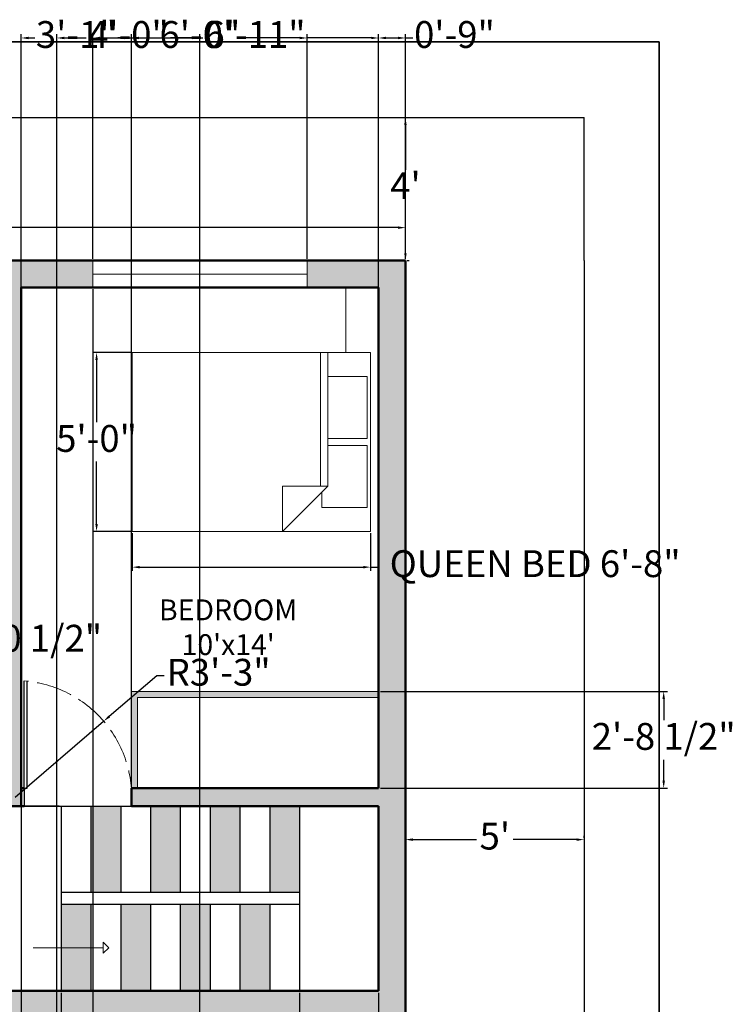
# Model space of a CAD drawing. Units: inches. Extents: x 24899 to 30135, y 37074 to 37745.
# Tile 3 of 3: x 25132 to 25371, y 37333 to 37663. Entities that reach past the tile are written whole.
import ezdxf

# ---------------------------------------------------------------- set-up
doc = ezdxf.new("R2010")
doc.units = ezdxf.units.IN
doc.linetypes.add('ACAD_ISO02W100', pattern=[15, 12, -3])
for name, color, linetype, lineweight in [('A-ANNO-DIMS', 2, 'Continuous', 18), ('A-ANNO-SYMB', 7, 'Continuous', 18), ('A-ANNO-TTLB', 7, 'Continuous', 35), ('A-AREA-IDEN', 7, 'Continuous', 25), ('A-DOOR', 4, 'Continuous', 25), ('A-DOOR-SWNG', 4, 'ACAD_ISO02W100', 13), ('A-FLOR-STRS', 7, 'Continuous', 25), ('A-FLOR-STRS-PATT', 8, 'Continuous', 13), ('A-FURN', 8, 'Continuous', 18), ('A-GLAZ', 4, 'Continuous', 18), ('A-WALL', 7, 'Continuous', 50), ('C-PROP', 3, 'Continuous', 25)]:
    doc.layers.add(name, color=color, linetype=linetype, lineweight=lineweight)
doc.layers.add('A-FURN-PATT', color=251, linetype='Continuous', lineweight=13, true_color=0x636466)
doc.layers.add('A-WALL-PATT', color=18, linetype='Continuous', lineweight=13, true_color=0x000000)
doc.styles.get("Standard").update_dxf_attribs({"font": 'arial.ttf'})
doc.dimstyles.new('ISO-25', dxfattribs={"dimtxt": 9, "dimasz": 2.5, "dimexe": 1.25, "dimexo": 0.625, "dimgap": 2, "dimtad": 0, "dimtih": 1, "dimtoh": 1, "dimdec": 1, "dimlunit": 4, "dimtxsty": 'Standard', "dimcen": 2.5, "dimadec": 0, "dimazin": 0, "dimtfac": 0.5, "dimtdec": 1, "dimtmove": 0, "dimatfit": 3, "dimfxl": 1, "dimarcsym": 0})

# ---------------------------------------------------------------- blocks, each defined once
blk = doc.blocks.new('*D1')
at = {"layer": 'A-ANNO-DIMS', "color": 0, "lineweight": -2, "transparency": 16777216}
for p, q in [((24949.48, 37583.06), (24949.48, 37594.75)), ((24951.98, 37593.5), (25095.76, 37593.5)), ((25258.98, 37593.5), (25115.19, 37593.5)), ((25261.48, 37583.06), (25261.48, 37594.75))]:
    blk.add_line(p, q, dxfattribs=at)
at = {"layer": 'A-ANNO-DIMS', "color": 0, "transparency": 16777216}
for points in [[(24951.98, 37593.92), (24951.98, 37593.09), (24949.48, 37593.5)], [(25258.98, 37593.92), (25258.98, 37593.09), (25261.48, 37593.5)]]:
    blk.add_solid(points, dxfattribs=at)
at = {"layer": 'Defpoints', "color": 0, "transparency": 16777216}
for p in [(25261.48, 37593.5), (24949.48, 37582.43), (25261.48, 37582.43)]:
    blk.add_point(p, dxfattribs=at)
at = {"layer": 'A-ANNO-DIMS', "color": 0, "transparency": 16777216, "insert": (25105.48, 37593.5), "char_height": 9, "attachment_point": 5}
blk.add_mtext("26'", dxfattribs=at)
blk = doc.blocks.new('*D7')
at = {"layer": 'A-ANNO-DIMS', "color": 0, "lineweight": -2, "transparency": 16777216}
for p, q in [((25261.48, 37388.81), (25261.48, 37389.44)), ((25263.98, 37388.19), (25285.34, 37388.19)), ((25318.98, 37388.19), (25297.62, 37388.19)), ((25321.48, 37388.81), (25321.48, 37389.44))]:
    blk.add_line(p, q, dxfattribs=at)
at = {"layer": 'A-ANNO-DIMS', "color": 0, "transparency": 16777216}
for points in [[(25263.98, 37388.6), (25263.98, 37387.77), (25261.48, 37388.19)], [(25318.98, 37388.6), (25318.98, 37387.77), (25321.48, 37388.19)]]:
    blk.add_solid(points, dxfattribs=at)
at = {"layer": 'Defpoints', "color": 0, "transparency": 16777216}
for p in [(25261.48, 37388.19), (25321.48, 37388.19), (25321.48, 37388.19)]:
    blk.add_point(p, dxfattribs=at)
at = {"layer": 'A-ANNO-DIMS', "color": 0, "transparency": 16777216, "insert": (25291.48, 37388.19), "char_height": 9, "attachment_point": 5}
blk.add_mtext("5'", dxfattribs=at)
blk = doc.blocks.new('*D8')
at = {"layer": 'A-ANNO-DIMS', "color": 0, "lineweight": -2, "transparency": 16777216}
for p, q in [((25262.1, 37630.43), (25262.73, 37630.43)), ((25261.48, 37627.93), (25261.48, 37612.93)), ((25261.48, 37584.93), (25261.48, 37599.93)), ((25262.1, 37582.43), (25262.73, 37582.43))]:
    blk.add_line(p, q, dxfattribs=at)
at = {"layer": 'A-ANNO-DIMS', "color": 0, "transparency": 16777216}
for points in [[(25261.06, 37627.93), (25261.89, 37627.93), (25261.48, 37630.43)], [(25261.06, 37584.93), (25261.89, 37584.93), (25261.48, 37582.43)]]:
    blk.add_solid(points, dxfattribs=at)
at = {"layer": 'Defpoints', "color": 0, "transparency": 16777216}
for p in [(25261.48, 37630.43), (25261.48, 37630.43), (25261.48, 37582.43)]:
    blk.add_point(p, dxfattribs=at)
at = {"layer": 'A-ANNO-DIMS', "color": 0, "transparency": 16777216, "insert": (25261.48, 37606.43), "char_height": 9, "attachment_point": 5}
blk.add_mtext("4'", dxfattribs=at)
blk = doc.blocks.new('Bed - Queen')
for p, q in [((0, -80.00003), (0, 0)), ((0, 0), (59.99999, 0)), ((59.99999, 0), (59.99999, -80.00003)), ((7.99999, -1.2), (28.79998, -1.2)), ((7.99999, -14.4), (7.99999, -1.2)), ((28.79998, -1.2), (28.79998, -14.4)), ((31.19999, -1.2), (51.99999, -1.2)), ((31.19999, -14.4), (31.19999, -1.2)), ((51.99999, -1.2), (51.99999, -16.4)), ((0, -14.4), (44.8, -14.4)), ((59.99999, -29.6), (44.8, -14.4)), ((44.8, -14.4), (44.8, -29.6)), ((51.99999, -16.4), (46.79936, -16.4)), ((44.8, -16.8), (0, -16.8)), ((44.8, -29.6), (59.99999, -29.6)), ((59.99999, -80.00003), (0, -80.00003))]:
    blk.add_line(p, q)
blk = doc.blocks.new('*D15')
at = {"layer": 'A-ANNO-DIMS', "color": 0, "lineweight": -2, "transparency": 16777216}
for p, q in [((25169.79, 37490.97), (25169.79, 37478.35)), ((25249.79, 37490.97), (25249.79, 37478.35)), ((25172.29, 37479.6), (25247.29, 37479.6)), ((25249.79, 37479.6), (25252.29, 37479.6))]:
    blk.add_line(p, q, dxfattribs=at)
at = {"layer": 'A-ANNO-DIMS', "color": 0, "transparency": 16777216}
for points in [[(25172.29, 37480.01), (25172.29, 37479.18), (25169.79, 37479.6)], [(25247.29, 37480.01), (25247.29, 37479.18), (25249.79, 37479.6)]]:
    blk.add_solid(points, dxfattribs=at)
at = {"layer": 'Defpoints', "color": 0, "transparency": 16777216}
for p in [(25169.79, 37491.6), (25249.79, 37491.6), (25249.79, 37479.6)]:
    blk.add_point(p, dxfattribs=at)
at = {"layer": 'A-ANNO-DIMS', "color": 0, "transparency": 16777216, "insert": (25305.02, 37479.6), "char_height": 9, "attachment_point": 5}
blk.add_mtext('QUEEN BED 6\'-8"', dxfattribs=at)
blk = doc.blocks.new('*D16')
at = {"layer": 'A-ANNO-DIMS', "color": 0, "lineweight": -2, "transparency": 16777216}
for p, q in [((25169.17, 37551.6), (25156.54, 37551.6)), ((25157.79, 37549.1), (25157.79, 37528.19)), ((25157.79, 37494.1), (25157.79, 37515)), ((25169.17, 37491.6), (25156.54, 37491.6))]:
    blk.add_line(p, q, dxfattribs=at)
at = {"layer": 'A-ANNO-DIMS', "color": 0, "transparency": 16777216}
for points in [[(25157.38, 37549.1), (25158.21, 37549.1), (25157.79, 37551.6)], [(25157.38, 37494.1), (25158.21, 37494.1), (25157.79, 37491.6)]]:
    blk.add_solid(points, dxfattribs=at)
at = {"layer": 'Defpoints', "color": 0, "transparency": 16777216}
for p in [(25169.79, 37551.6), (25157.79, 37491.6), (25169.79, 37491.6)]:
    blk.add_point(p, dxfattribs=at)
at = {"layer": 'A-ANNO-DIMS', "color": 0, "transparency": 16777216, "insert": (25157.79, 37521.6), "char_height": 9, "attachment_point": 5}
blk.add_mtext('5\'-0"', dxfattribs=at)
blk = doc.blocks.new('*D22')
at = {"layer": 'A-ANNO-DIMS', "color": 0, "lineweight": -2, "transparency": 16777216}
for p, q in [((25087.48, 37572.81), (25087.48, 37086.48)), ((25111.48, 37572.81), (25111.48, 37086.48)), ((25089.98, 37087.73), (25108.98, 37087.73)), ((25111.48, 37087.73), (25113.98, 37087.73))]:
    blk.add_line(p, q, dxfattribs=at)
at = {"layer": 'A-ANNO-DIMS', "color": 0, "transparency": 16777216}
for points in [[(25089.98, 37088.15), (25089.98, 37087.32), (25087.48, 37087.73)], [(25108.98, 37088.15), (25108.98, 37087.32), (25111.48, 37087.73)]]:
    blk.add_solid(points, dxfattribs=at)
at = {"layer": 'Defpoints', "color": 0, "transparency": 16777216}
for p in [(25087.48, 37573.43), (25111.48, 37573.43), (25111.48, 37087.73)]:
    blk.add_point(p, dxfattribs=at)
at = {"layer": 'A-ANNO-DIMS', "color": 0, "transparency": 16777216, "insert": (25128.02, 37087.73), "char_height": 9, "attachment_point": 5}
blk.add_mtext('2\'-0"', dxfattribs=at)
blk = doc.blocks.new('*D23')
at = {"layer": 'A-ANNO-DIMS', "color": 0, "lineweight": -2, "transparency": 16777216}
for p, q in [((25132.48, 37572.81), (25132.48, 37086.48)), ((25156.48, 37572.81), (25156.48, 37086.48)), ((25134.98, 37087.73), (25153.98, 37087.73)), ((25156.48, 37087.73), (25158.98, 37087.73))]:
    blk.add_line(p, q, dxfattribs=at)
at = {"layer": 'A-ANNO-DIMS', "color": 0, "transparency": 16777216}
for points in [[(25134.98, 37088.15), (25134.98, 37087.32), (25132.48, 37087.73)], [(25153.98, 37088.15), (25153.98, 37087.32), (25156.48, 37087.73)]]:
    blk.add_solid(points, dxfattribs=at)
at = {"layer": 'Defpoints', "color": 0, "transparency": 16777216}
for p in [(25132.48, 37573.43), (25156.48, 37573.43), (25156.48, 37087.73)]:
    blk.add_point(p, dxfattribs=at)
at = {"layer": 'A-ANNO-DIMS', "color": 0, "transparency": 16777216, "insert": (25173.02, 37087.73), "char_height": 9, "attachment_point": 5}
blk.add_mtext('2\'-0"', dxfattribs=at)
blk = doc.blocks.new('*D24')
at = {"layer": 'A-ANNO-DIMS', "color": 0, "lineweight": -2, "transparency": 16777216}
for p, q in [((25156.48, 37583.06), (25156.48, 37658.38)), ((25228.48, 37583.06), (25228.48, 37658.38)), ((25158.98, 37657.13), (25178.49, 37657.13)), ((25225.98, 37657.13), (25206.46, 37657.13))]:
    blk.add_line(p, q, dxfattribs=at)
at = {"layer": 'A-ANNO-DIMS', "color": 0, "transparency": 16777216}
for points in [[(25158.98, 37657.55), (25158.98, 37656.72), (25156.48, 37657.13)], [(25225.98, 37657.55), (25225.98, 37656.72), (25228.48, 37657.13)]]:
    blk.add_solid(points, dxfattribs=at)
at = {"layer": 'Defpoints', "color": 0, "transparency": 16777216}
for p in [(25228.48, 37657.13), (25156.48, 37582.43), (25228.48, 37582.43)]:
    blk.add_point(p, dxfattribs=at)
at = {"layer": 'A-ANNO-DIMS', "color": 0, "transparency": 16777216, "insert": (25192.48, 37657.13), "char_height": 9, "attachment_point": 5}
blk.add_mtext('6\'-0"', dxfattribs=at)
blk = doc.blocks.new('*D29')
at = {"layer": 'A-ANNO-DIMS', "color": 0, "lineweight": -2, "transparency": 16777216}
for p, q in [((25132.48, 37406.06), (25132.48, 37658.38)), ((25169.48, 37406.06), (25169.48, 37658.38)), ((25134.98, 37657.13), (25137.02, 37657.13)), ((25166.98, 37657.13), (25164.94, 37657.13))]:
    blk.add_line(p, q, dxfattribs=at)
at = {"layer": 'A-ANNO-DIMS', "color": 0, "transparency": 16777216}
for points in [[(25134.98, 37657.55), (25134.98, 37656.72), (25132.48, 37657.13)], [(25166.98, 37657.55), (25166.98, 37656.72), (25169.48, 37657.13)]]:
    blk.add_solid(points, dxfattribs=at)
at = {"layer": 'Defpoints', "color": 0, "transparency": 16777216}
for p in [(25169.48, 37657.13), (25132.48, 37405.43), (25169.48, 37405.43)]:
    blk.add_point(p, dxfattribs=at)
at = {"layer": 'A-ANNO-DIMS', "color": 0, "transparency": 16777216, "insert": (25150.98, 37657.13), "char_height": 9, "attachment_point": 5}
blk.add_mtext('3\'-1"', dxfattribs=at)
blk = doc.blocks.new('*D30')
at = {"layer": 'A-ANNO-DIMS', "color": 0, "lineweight": -2, "transparency": 16777216}
for p, q in [((25145.9, 37336.81), (25145.9, 37086.48)), ((25225.9, 37336.81), (25225.9, 37086.48)), ((25148.4, 37087.73), (25171.91, 37087.73)), ((25223.4, 37087.73), (25199.89, 37087.73))]:
    blk.add_line(p, q, dxfattribs=at)
at = {"layer": 'A-ANNO-DIMS', "color": 0, "transparency": 16777216}
for points in [[(25148.4, 37088.15), (25148.4, 37087.32), (25145.9, 37087.73)], [(25223.4, 37088.15), (25223.4, 37087.32), (25225.9, 37087.73)]]:
    blk.add_solid(points, dxfattribs=at)
at = {"layer": 'Defpoints', "color": 0, "transparency": 16777216}
for p in [(25145.9, 37337.43), (25225.9, 37337.43), (25225.9, 37087.73)]:
    blk.add_point(p, dxfattribs=at)
at = {"layer": 'A-ANNO-DIMS', "color": 0, "transparency": 16777216, "insert": (25185.9, 37087.73), "char_height": 9, "attachment_point": 5}
blk.add_mtext('6\'-8"', dxfattribs=at)
blk = doc.blocks.new('*D31')
at = {"layer": 'A-ANNO-DIMS', "color": 0, "lineweight": -2, "transparency": 16777216}
for p, q in [((25225.9, 37336.81), (25225.9, 37086.48)), ((25252.48, 37336.81), (25252.48, 37086.48)), ((25228.4, 37087.73), (25249.98, 37087.73)), ((25252.48, 37087.73), (25254.98, 37087.73))]:
    blk.add_line(p, q, dxfattribs=at)
at = {"layer": 'A-ANNO-DIMS', "color": 0, "transparency": 16777216}
for points in [[(25228.4, 37088.15), (25228.4, 37087.32), (25225.9, 37087.73)], [(25249.98, 37088.15), (25249.98, 37087.32), (25252.48, 37087.73)]]:
    blk.add_solid(points, dxfattribs=at)
at = {"layer": 'Defpoints', "color": 0, "transparency": 16777216}
for p in [(25225.9, 37337.43), (25252.48, 37337.43), (25252.48, 37087.73)]:
    blk.add_point(p, dxfattribs=at)
at = {"layer": 'A-ANNO-DIMS', "color": 0, "transparency": 16777216, "insert": (25279.5, 37087.73), "char_height": 9, "attachment_point": 5}
blk.add_mtext('2\'-2 1/2"', dxfattribs=at)
blk = doc.blocks.new('*D32')
at = {"layer": 'A-ANNO-DIMS', "color": 0, "lineweight": -2, "transparency": 16777216}
for p, q in [((25145.27, 37399.43), (24921.53, 37399.43)), ((24922.78, 37396.93), (24922.78, 37375.03)), ((24922.78, 37339.93), (24922.78, 37361.84)), ((25145.27, 37337.43), (24921.53, 37337.43))]:
    blk.add_line(p, q, dxfattribs=at)
at = {"layer": 'A-ANNO-DIMS', "color": 0, "transparency": 16777216}
for points in [[(24922.36, 37396.93), (24923.19, 37396.93), (24922.78, 37399.43)], [(24922.36, 37339.93), (24923.19, 37339.93), (24922.78, 37337.43)]]:
    blk.add_solid(points, dxfattribs=at)
at = {"layer": 'Defpoints', "color": 0, "transparency": 16777216}
for p in [(24922.78, 37399.43), (25145.9, 37399.43), (25145.9, 37337.43)]:
    blk.add_point(p, dxfattribs=at)
at = {"layer": 'A-ANNO-DIMS', "color": 0, "transparency": 16777216, "insert": (24922.78, 37368.43), "char_height": 9, "attachment_point": 5}
blk.add_mtext('5\'-2"', dxfattribs=at)
blk = doc.blocks.new('*D33')
at = {"layer": 'A-ANNO-DIMS', "color": 0, "lineweight": -2, "transparency": 16777216}
for p, q in [((25144.48, 37184.06), (25144.48, 37658.38)), ((25192.48, 37184.06), (25192.48, 37658.38)), ((25146.98, 37657.13), (25154.33, 37657.13)), ((25189.98, 37657.13), (25182.62, 37657.13))]:
    blk.add_line(p, q, dxfattribs=at)
at = {"layer": 'A-ANNO-DIMS', "color": 0, "transparency": 16777216}
for points in [[(25146.98, 37657.55), (25146.98, 37656.72), (25144.48, 37657.13)], [(25189.98, 37657.55), (25189.98, 37656.72), (25192.48, 37657.13)]]:
    blk.add_solid(points, dxfattribs=at)
at = {"layer": 'Defpoints', "color": 0, "transparency": 16777216}
for p in [(25192.48, 37657.13), (25144.48, 37183.43), (25192.48, 37183.43)]:
    blk.add_point(p, dxfattribs=at)
at = {"layer": 'A-ANNO-DIMS', "color": 0, "transparency": 16777216, "insert": (25168.48, 37657.13), "char_height": 9, "attachment_point": 5}
blk.add_mtext('4\'-0"', dxfattribs=at)
blk = doc.blocks.new('*D42')
at = {"layer": 'A-ANNO-DIMS', "color": 0, "lineweight": -2, "transparency": 16777216}
for p, q in [((25169.48, 37406.06), (25169.48, 37658.38)), ((25252.48, 37406.06), (25252.48, 37658.38)), ((25171.98, 37657.13), (25193.49, 37657.13)), ((25249.98, 37657.13), (25228.46, 37657.13))]:
    blk.add_line(p, q, dxfattribs=at)
at = {"layer": 'A-ANNO-DIMS', "color": 0, "transparency": 16777216}
for points in [[(25171.98, 37657.55), (25171.98, 37656.72), (25169.48, 37657.13)], [(25249.98, 37657.55), (25249.98, 37656.72), (25252.48, 37657.13)]]:
    blk.add_solid(points, dxfattribs=at)
at = {"layer": 'Defpoints', "color": 0, "transparency": 16777216}
for p in [(25252.48, 37657.13), (25169.48, 37405.43), (25252.48, 37405.43)]:
    blk.add_point(p, dxfattribs=at)
at = {"layer": 'A-ANNO-DIMS', "color": 0, "transparency": 16777216, "insert": (25210.98, 37657.13), "char_height": 9, "attachment_point": 5}
blk.add_mtext('6\'-11"', dxfattribs=at)
blk = doc.blocks.new('*D43')
at = {"layer": 'A-ANNO-DIMS', "color": 0, "lineweight": -2, "transparency": 16777216}
for p, q in [((25253.1, 37437.87), (25349.43, 37437.87)), ((25348.18, 37435.37), (25348.18, 37428.3)), ((25348.18, 37407.93), (25348.18, 37415)), ((25253.1, 37405.43), (25349.43, 37405.43))]:
    blk.add_line(p, q, dxfattribs=at)
at = {"layer": 'A-ANNO-DIMS', "color": 0, "transparency": 16777216}
for points in [[(25347.76, 37435.37), (25348.59, 37435.37), (25348.18, 37437.87)], [(25347.76, 37407.93), (25348.59, 37407.93), (25348.18, 37405.43)]]:
    blk.add_solid(points, dxfattribs=at)
at = {"layer": 'Defpoints', "color": 0, "transparency": 16777216}
for p in [(25252.48, 37437.87), (25348.18, 37437.87), (25252.48, 37405.43)]:
    blk.add_point(p, dxfattribs=at)
at = {"layer": 'A-ANNO-DIMS', "color": 0, "transparency": 16777216, "insert": (25348.18, 37421.65), "char_height": 9, "attachment_point": 5}
blk.add_mtext('2\'-8 1/2"', dxfattribs=at)
blk = doc.blocks.new('*D44')
at = {"layer": 'A-ANNO-DIMS', "color": 0, "lineweight": -2, "transparency": 16777216}
for p, q in [((25252.48, 37574.06), (25252.48, 37658.38)), ((25261.48, 37583.06), (25261.48, 37658.38)), ((25254.98, 37657.13), (25258.98, 37657.13)), ((25261.48, 37657.13), (25263.98, 37657.13))]:
    blk.add_line(p, q, dxfattribs=at)
at = {"layer": 'A-ANNO-DIMS', "color": 0, "transparency": 16777216}
for points in [[(25254.98, 37657.55), (25254.98, 37656.72), (25252.48, 37657.13)], [(25258.98, 37657.55), (25258.98, 37656.72), (25261.48, 37657.13)]]:
    blk.add_solid(points, dxfattribs=at)
at = {"layer": 'Defpoints', "color": 0, "transparency": 16777216}
for p in [(25261.48, 37657.13), (25261.48, 37582.43), (25252.48, 37573.43)]:
    blk.add_point(p, dxfattribs=at)
at = {"layer": 'A-ANNO-DIMS', "color": 0, "transparency": 16777216, "insert": (25277.94, 37657.13), "char_height": 9, "attachment_point": 5}
blk.add_mtext('0\'-9"', dxfattribs=at)
blk = doc.blocks.new('*D47')
at = {"layer": 'A-ANNO-DIMS', "color": 0, "lineweight": -2, "transparency": 16777216}
for p, q in [((25177.99, 37443.16), (25162.07, 37429.52)), ((25180.49, 37443.16), (25177.99, 37443.16)), ((25130.48, 37402.43), (25160.17, 37427.89))]:
    blk.add_line(p, q, dxfattribs=at)
at = {"layer": 'A-ANNO-DIMS', "color": 0, "transparency": 16777216}
blk.add_solid([(25161.8, 37429.83), (25162.34, 37429.2), (25160.17, 37427.89)], dxfattribs=at)
at = {"layer": 'Defpoints', "color": 0, "transparency": 16777216}
for p in [(25160.17, 37427.89), (25130.48, 37402.43)]:
    blk.add_point(p, dxfattribs=at)
at = {"layer": 'A-ANNO-DIMS', "color": 0, "transparency": 16777216, "insert": (25198.76, 37443.16), "char_height": 9, "attachment_point": 5}
blk.add_mtext('R3\'-3"', dxfattribs=at)
blk = doc.blocks.new('*D50')
at = {"layer": 'A-ANNO-DIMS', "color": 0, "lineweight": -2, "transparency": 16777216}
for p, q in [((25075.33, 37454.58), (25072.83, 37454.58)), ((25077.83, 37454.58), (25088.11, 37454.58)), ((25093.11, 37454.58), (25090.61, 37454.58))]:
    blk.add_line(p, q, dxfattribs=at)
at = {"layer": 'A-ANNO-DIMS', "color": 0, "transparency": 16777216}
for points in [[(25075.33, 37454.99), (25075.33, 37454.16), (25077.83, 37454.58)], [(25090.61, 37455), (25090.61, 37454.16), (25088.11, 37454.58)]]:
    blk.add_solid(points, dxfattribs=at)
at = {"layer": 'Defpoints', "color": 0, "transparency": 16777216}
for p in [(25077.83, 37454.58), (25088.11, 37454.58)]:
    blk.add_point(p, dxfattribs=at)
at = {"layer": 'A-ANNO-DIMS', "color": 0, "transparency": 16777216, "insert": (25125.95, 37454.58), "char_height": 9, "attachment_point": 5}
blk.add_mtext('∅0\'-10 1/2"', dxfattribs=at)

msp = doc.modelspace()

# ---------------------------------------------------------------- hatches: boundary and pattern name
at = {"layer": 'A-FLOR-STRS-PATT'}
h = msp.add_hatch(color=256, dxfattribs=at)
h.dxf.hatch_style = 1
h.paths.add_polyline_path([(25155.9, 37366.43), (25145.9, 37366.43), (25145.9, 37351.93), (25155.9, 37351.93)])
h.paths.add_polyline_path([(25155.9, 37351.93), (25145.9, 37351.93), (25145.9, 37337.43), (25155.9, 37337.43)])
h.paths.add_polyline_path([(25175.9, 37366.43), (25165.9, 37366.43), (25165.9, 37337.43), (25175.9, 37337.43)])
h.paths.add_polyline_path([(25195.9, 37366.43), (25185.9, 37366.43), (25185.9, 37337.43), (25195.9, 37337.43)])
h.paths.add_polyline_path([(25215.9, 37366.43), (25205.9, 37366.43), (25205.9, 37337.43), (25215.9, 37337.43)])
h.paths.add_polyline_path([(25225.9, 37399.43), (25215.9, 37399.43), (25215.9, 37370.43), (25225.9, 37370.43)])
h.paths.add_polyline_path([(25205.9, 37399.43), (25195.9, 37399.43), (25195.9, 37370.43), (25205.9, 37370.43)])
h.paths.add_polyline_path([(25185.9, 37399.43), (25175.9, 37399.43), (25175.9, 37370.43), (25185.9, 37370.43)])
h.paths.add_polyline_path([(25165.9, 37399.43), (25155.9, 37399.43), (25155.9, 37370.43), (25165.9, 37370.43)])
at = {"layer": 'A-FURN-PATT'}
h = msp.add_hatch(color=256, dxfattribs=at)
h.dxf.hatch_style = 1
h.paths.add_polyline_path([(25171.48, 37435.87), (25252.48, 37435.87), (25252.48, 37437.87), (25169.48, 37437.87), (25169.48, 37405.43), (25171.48, 37405.43)])
at = {"layer": 'A-WALL-PATT'}
h = msp.add_hatch(color=256, dxfattribs=at)
h.dxf.hatch_style = 1
h.paths.add_polyline_path([(25261.48, 37582.43), (25228.48, 37582.43), (25228.48, 37573.43), (25252.48, 37573.43), (25252.48, 37405.43), (25169.48, 37405.43, -0.038405), (25169.48, 37399.43), (25252.48, 37399.43), (25252.48, 37337.43), (25201.48, 37337.43), (24958.48, 37337.43), (24958.48, 37465.43), (24988.48, 37465.43), (24988.48, 37471.43), (24958.48, 37471.43), (24958.48, 37573.43), (24994.48, 37573.43), (24994.48, 37582.43), (24949.48, 37582.43), (24949.48, 37174.43), (25144.48, 37174.43, -0.042779), (25144.48, 37183.43), (24958.48, 37183.43), (24958.48, 37328.43), (25192.48, 37328.43), (25192.48, 37183.43), (25192.48, 37174.43), (25201.48, 37174.43), (25201.48, 37183.43), (25201.48, 37328.43), (25261.48, 37328.43)])
h.paths.add_polyline_path([(25087.48, 37582.43), (25030.48, 37582.43, -0.077125), (25030.48, 37573.43), (25066.48, 37573.43), (25066.48, 37471.43), (25036.48, 37471.43), (25036.48, 37465.43), (25066.48, 37465.43), (25066.48, 37430.04), (25095.6, 37430.04), (25095.6, 37435.01), (25072.48, 37435.01), (25072.48, 37465.43), (25072.48, 37471.43), (25095.48, 37471.43, -0.045361), (25095.48, 37477.43), (25072.48, 37477.43), (25072.48, 37573.43), (25087.48, 37573.43)], flags=0)
h.paths.add_polyline_path([(25156.48, 37582.43), (25111.48, 37582.43), (25111.48, 37573.43), (25126.48, 37573.43), (25126.48, 37477.43), (25126.48, 37471.43), (25126.48, 37399.43), (25132.48, 37399.43), (25132.48, 37405.43), (25132.48, 37471.43), (25132.48, 37573.43), (25156.48, 37573.43)], flags=17)

# ---------------------------------------------------------------- linework, layer by layer
at = {"layer": 'A-ANNO-SYMB'}
for p, q in [((25155.9, 37351.93), (25136.45, 37351.93)), ((25155.9, 37351.93), (25160.05, 37351.93)), ((25160.05, 37351.93), (25160.02, 37353.77)), ((25160.02, 37353.77), (25161.89, 37351.9)), ((25160.04, 37350.05), (25160.05, 37351.93)), ((25161.89, 37351.9), (25160.04, 37350.05))]:
    msp.add_line(p, q, dxfattribs=at)
at = {"layer": 'A-ANNO-TTLB'}
msp.add_lwpolyline([(24909.5, 37655.83), (25346.61, 37655.83), (25346.61, 37086.99), (24909.5, 37086.99)], close=True, dxfattribs=at)
at = {"layer": 'A-DOOR'}
for p, q in [((25133.48, 37405.43), (25133.48, 37441.43)), ((25134.48, 37405.43), (25134.48, 37441.43)), ((25133.48, 37405.43), (25133.48, 37399.43)), ((25133.48, 37405.43), (25134.48, 37405.43)), ((25133.48, 37399.43), (25169.48, 37399.43))]:
    msp.add_line(p, q, dxfattribs=at)
at = {"layer": 'A-DOOR-SWNG'}
msp.add_arc((25130.48, 37402.43), 39.12, 355.6013, 85.6013, dxfattribs=at)
at = {"layer": 'A-FLOR-STRS'}
for p, q in [((25145.9, 37399.43), (25145.9, 37337.43)), ((25155.9, 37399.43), (25155.9, 37370.43)), ((25165.9, 37399.43), (25165.9, 37370.43)), ((25175.9, 37399.43), (25175.9, 37370.43)), ((25185.9, 37399.43), (25185.9, 37370.43)), ((25195.9, 37399.43), (25195.9, 37370.43)), ((25205.9, 37399.43), (25205.9, 37370.43)), ((25215.9, 37399.43), (25215.9, 37370.43)), ((25225.9, 37399.43), (25225.9, 37337.43)), ((25225.9, 37370.43), (25145.9, 37370.43)), ((25225.9, 37366.43), (25145.9, 37366.43)), ((25155.9, 37366.43), (25155.9, 37337.43)), ((25165.9, 37366.43), (25165.9, 37337.43)), ((25175.9, 37366.43), (25175.9, 37337.43)), ((25185.9, 37366.43), (25185.9, 37337.43)), ((25195.9, 37366.43), (25195.9, 37337.43)), ((25205.9, 37366.43), (25205.9, 37337.43)), ((25215.9, 37366.43), (25215.9, 37337.43))]:
    msp.add_line(p, q, dxfattribs=at)
at = {"layer": 'A-FURN'}
for p, q in [((25241.52, 37573.43), (25241.52, 37551.6)), ((25252.48, 37437.87), (25169.48, 37437.87)), ((25169.48, 37405.43), (25169.48, 37437.87)), ((25252.48, 37435.87), (25171.48, 37435.87)), ((25171.48, 37405.43), (25171.48, 37435.87))]:
    msp.add_line(p, q, dxfattribs=at)
at = {"layer": 'A-GLAZ'}
for p, q in [((25156.48, 37573.43), (25156.48, 37582.43)), ((25228.48, 37573.43), (25228.48, 37582.43)), ((25156.48, 37577.93), (25228.48, 37577.93))]:
    msp.add_line(p, q, dxfattribs=at)
at = {"layer": 'A-WALL'}
for p, q in [((25030.48, 37582.43), (25261.48, 37582.43)), ((25261.48, 37328.43), (25261.48, 37582.43)), ((25132.48, 37573.43), (25132.48, 37471.43)), ((25132.48, 37573.43), (25252.48, 37573.43)), ((25252.48, 37405.43), (25252.48, 37573.43)), ((25132.48, 37471.43), (25132.48, 37405.43)), ((25132.48, 37405.43), (25133.48, 37405.43)), ((25132.48, 37405.43), (25132.48, 37399.43)), ((25169.48, 37405.43), (25169.48, 37399.43)), ((25169.48, 37405.43), (25252.48, 37405.43)), ((25132.48, 37399.43), (25126.48, 37399.43)), ((25132.48, 37399.43), (25133.48, 37399.43)), ((25169.48, 37399.43), (25252.48, 37399.43)), ((25252.48, 37337.43), (25252.48, 37399.43)), ((24958.48, 37337.43), (25201.48, 37337.43)), ((25201.48, 37337.43), (25252.48, 37337.43))]:
    msp.add_line(p, q, dxfattribs=at)
at = {"layer": 'C-PROP'}
for p, q in [((24949.48, 37630.43), (25321.48, 37630.43)), ((25321.48, 37582.43), (25321.48, 37630.43)), ((25321.48, 37582.43), (25321.48, 37114.43))]:
    msp.add_line(p, q, dxfattribs=at)

# ---------------------------------------------------------------- block references
at = {"layer": 'A-FURN', "rotation": 270}
msp.add_blockref('Bed - Queen', (25249.79, 37551.6), dxfattribs=at)

# ---------------------------------------------------------------- texts
at = {"layer": 'A-AREA-IDEN', "insert": (25167.93, 37468.77), "char_height": 7, "attachment_point": 1}
msp.add_mtext_dynamic_manual_height_columns("\\pxqc;{\\fArial|b1|i0|c0|p34;BEDROOM\\P10'x14'}", width=68.0767, gutter_width=12.5, heights=[0], dxfattribs=at)

# ---------------------------------------------------------------- dimensions: what is measured, and where the dimension line sits
at = {"layer": 'A-ANNO-DIMS'}
for base, p1, p2, override, picture, middle in [((25169.48, 37657.13), (25132.48, 37405.43), (25169.48, 37405.43), {"dimdec": 1, "dimlfac": 1, "dimrnd": 0, "dimzin": 1, "dimdsep": 46, "dimlunit": 4, "dimfrac": 2}, '*D29', (25150.98, 37657.13)), ((25192.48, 37657.13), (25144.48, 37183.43), (25192.48, 37183.43), {"dimdec": 1, "dimlfac": 1, "dimrnd": 0, "dimzin": 1, "dimdsep": 46, "dimlunit": 4, "dimfrac": 2}, '*D33', (25168.48, 37657.13)), ((25228.48, 37657.13), (25156.48, 37582.43), (25228.48, 37582.43), {"dimdec": 1, "dimlfac": 1, "dimrnd": 0, "dimzin": 1, "dimdsep": 46, "dimlunit": 4, "dimfrac": 2}, '*D24', (25192.48, 37657.13)), ((25252.48, 37657.13), (25169.48, 37405.43), (25252.48, 37405.43), {"dimdec": 1, "dimlfac": 1, "dimrnd": 0, "dimzin": 1, "dimdsep": 46, "dimlunit": 4, "dimfrac": 2}, '*D42', (25210.98, 37657.13)), ((25261.48, 37657.13), (25252.48, 37573.43), (25261.48, 37582.43), {"dimdec": 1, "dimlfac": 1, "dimrnd": 0, "dimzin": 1, "dimdsep": 46, "dimlunit": 4, "dimfrac": 2}, '*D44', (25277.94, 37657.13)), ((25261.48, 37593.5), (24949.48, 37582.43), (25261.48, 37582.43), {"dimclrd": 0, "dimclre": 0, "dimclrt": 0}, '*D1', (25105.48, 37593.5)), ((25111.48, 37087.73), (25087.48, 37573.43), (25111.48, 37573.43), {"dimdec": 1, "dimlfac": 1, "dimrnd": 0, "dimzin": 1, "dimdsep": 46, "dimlunit": 4, "dimfrac": 2}, '*D22', (25128.02, 37087.73)), ((25156.48, 37087.73), (25132.48, 37573.43), (25156.48, 37573.43), {"dimdec": 1, "dimlfac": 1, "dimrnd": 0, "dimzin": 1, "dimdsep": 46, "dimlunit": 4, "dimfrac": 2}, '*D23', (25173.02, 37087.73)), ((25225.9, 37087.73), (25145.9, 37337.43), (25225.9, 37337.43), {"dimdec": 1, "dimlfac": 1, "dimrnd": 0, "dimzin": 1, "dimdsep": 46, "dimlunit": 4, "dimfrac": 2}, '*D30', (25185.9, 37087.73)), ((25252.48, 37087.73), (25225.9, 37337.43), (25252.48, 37337.43), {"dimdec": 1, "dimlfac": 1, "dimrnd": 0, "dimzin": 1, "dimdsep": 46, "dimlunit": 4, "dimfrac": 2}, '*D31', (25279.5, 37087.73))]:
    dim = msp.add_linear_dim(base=base, p1=p1, p2=p2, dimstyle='ISO-25', override=override, dxfattribs=at)
    dim.commit()
    dim.dimension.update_dxf_attribs({"geometry": picture, "text_midpoint": middle})
for base, p1, p2, angle, override, picture, middle in [((25261.48, 37630.43), (25261.48, 37582.43), (25261.48, 37630.43), 90, {"dimclrd": 0, "dimclre": 0, "dimclrt": 0}, '*D8', (25261.48, 37606.43)), ((25157.79, 37491.6), (25169.79, 37551.6), (25169.79, 37491.6), 270, {"dimdec": 1, "dimlfac": 1, "dimrnd": 0, "dimzin": 1, "dimdsep": 46, "dimlunit": 4, "dimfrac": 2}, '*D16', (25157.79, 37521.6)), ((25348.18, 37437.87), (25252.48, 37405.43), (25252.48, 37437.87), 90, {"dimdec": 1, "dimlfac": 1, "dimrnd": 0, "dimzin": 1, "dimdsep": 46, "dimlunit": 4, "dimfrac": 2}, '*D43', (25348.18, 37421.65)), ((24922.78, 37399.43), (25145.9, 37337.43), (25145.9, 37399.43), 90, {"dimdec": 1, "dimlfac": 1, "dimrnd": 0, "dimzin": 1, "dimdsep": 46, "dimlunit": 4, "dimfrac": 2}, '*D32', (24922.78, 37368.43)), ((25321.48, 37388.19), (25261.48, 37388.19), (25321.48, 37388.19), 180, {"dimclrd": 0, "dimclre": 0, "dimclrt": 0}, '*D7', (25291.48, 37388.19))]:
    dim = msp.add_linear_dim(base=base, p1=p1, p2=p2, angle=angle, dimstyle='ISO-25', override=override, dxfattribs=at)
    dim.commit()
    dim.dimension.update_dxf_attribs({"geometry": picture, "text_midpoint": middle})
dim = msp.add_linear_dim(base=(25249.79, 37479.6), p1=(25169.79, 37491.6), p2=(25249.79, 37491.6), text='QUEEN BED <>', dimstyle='ISO-25', override={"dimdec": 1, "dimlfac": 1, "dimrnd": 0, "dimzin": 1, "dimdsep": 46, "dimlunit": 4, "dimfrac": 2}, dxfattribs=at)
dim.commit()
dim.dimension.update_dxf_attribs({"geometry": '*D15', "text_midpoint": (25305.02, 37479.6)})
dim = msp.add_diameter_dim_2p(p1=(25077.83, 37454.58), p2=(25088.11, 37454.58), dimstyle='ISO-25', override={"dimdec": 1, "dimlfac": 1, "dimrnd": 0, "dimzin": 1, "dimdsep": 46, "dimlunit": 4, "dimfrac": 2}, dxfattribs=at)
dim.commit()
dim.dimension.update_dxf_attribs({"geometry": '*D50', "text_midpoint": (25093.11, 37454.58), "dimtype": 163})
dim = msp.add_radius_dim(center=(25130.48, 37402.43), mpoint=(25160.17, 37427.89), dimstyle='ISO-25', override={"dimdec": 1, "dimlfac": 1, "dimrnd": 0, "dimzin": 1, "dimdsep": 46, "dimlunit": 4, "dimfrac": 2}, dxfattribs=at)
dim.commit()
dim.dimension.update_dxf_attribs({"geometry": '*D47', "text_midpoint": (25198.76, 37443.16), "dimtype": 164})

doc.saveas('drawing.dxf')
